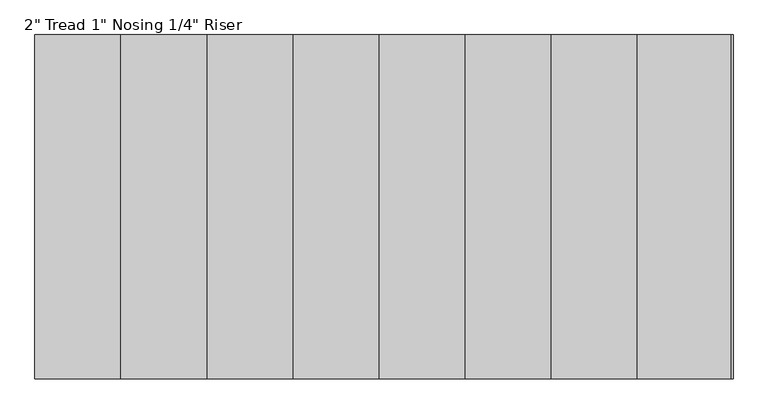
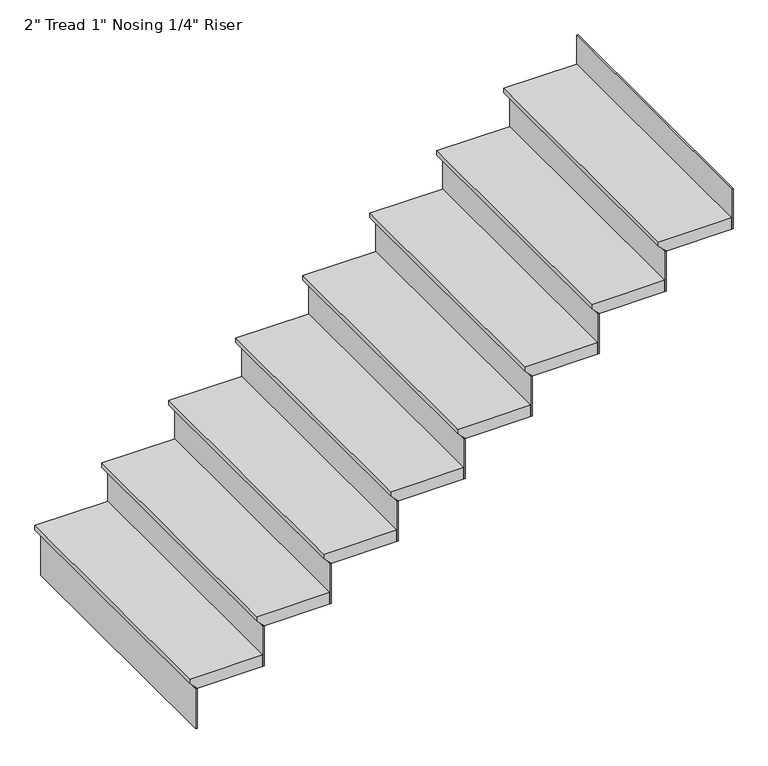
"""IFC4 building model written with IfcOpenShell, lengths in millimetres: stair flight geometry."""

from ifc_helpers import new_model, si_unit, frame, origin, place, context, project, spatial, polyline, outline, extrude, source, transform, mapped, element, save


def stair_flight_ef2f52e6(model_context):
    return source(origin(), model_context, "Body", "SweptSolid", [
        extrude(outline(polyline([(1778.0, -9891.2683044), (1778.0, -10196.0683044), (1758.95, -10196.0683044), (1733.55, -10170.6683044), (1727.2, -10170.6683044), (1727.2, -9891.2683044), (1778.0, -9891.2683044)])), frame((0.0, -2492.1891189, 0.0), z_axis=(0.0, 1.0, 0.0), x_axis=(0.0, 0.0, 1.0)), (0.0, 0.0, 1.0), 1117.6),
        extrude(outline(polyline([(-10164.3183044, -2492.1891189), (-10170.6683044, -2492.1891189), (-10170.6683044, -1374.5891189), (-10164.3183044, -1374.5891189), (-10164.3183044, -2492.1891189)])), frame((0.0, 0.0, 1549.4), z_axis=(0.0, 0.0, 1.0), x_axis=(1.0, 0.0, 0.0)), (0.0, 0.0, 1.0), 177.8),
        extrude(outline(polyline([(-9884.9183044, -2492.1891189), (-9891.2683044, -2492.1891189), (-9891.2683044, -1374.5891189), (-9884.9183044, -1374.5891189), (-9884.9183044, -2492.1891189)])), frame((0.0, 0.0, 1727.2), z_axis=(0.0, 0.0, 1.0), x_axis=(1.0, 0.0, 0.0)), (0.0, 0.0, 1.0), 177.8),
        extrude(outline(polyline([(1955.8, -9611.8683044), (1955.8, -9916.6683044), (1936.75, -9916.6683044), (1911.35, -9891.2683044), (1905.0, -9891.2683044), (1905.0, -9611.8683044), (1955.8, -9611.8683044)])), frame((0.0, -2492.1891189, 0.0), z_axis=(0.0, 1.0, 0.0), x_axis=(0.0, 0.0, 1.0)), (0.0, 0.0, 1.0), 1117.6),
        extrude(outline(polyline([(-9605.5183044, -2492.1891189), (-9611.8683044, -2492.1891189), (-9611.8683044, -1374.5891189), (-9605.5183044, -1374.5891189), (-9605.5183044, -2492.1891189)])), frame((0.0, 0.0, 1905.0), z_axis=(0.0, 0.0, 1.0), x_axis=(1.0, 0.0, 0.0)), (0.0, 0.0, 1.0), 177.8),
        extrude(outline(polyline([(2133.6, -9332.4683044), (2133.6, -9637.2683044), (2114.55, -9637.2683044), (2089.15, -9611.8683044), (2082.8, -9611.8683044), (2082.8, -9332.4683044), (2133.6, -9332.4683044)])), frame((0.0, -2492.1891189, 0.0), z_axis=(0.0, 1.0, 0.0), x_axis=(0.0, 0.0, 1.0)), (0.0, 0.0, 1.0), 1117.6),
        extrude(outline(polyline([(-9326.1183044, -2492.1891189), (-9332.4683044, -2492.1891189), (-9332.4683044, -1374.5891189), (-9326.1183044, -1374.5891189), (-9326.1183044, -2492.1891189)])), frame((0.0, 0.0, 2082.8), z_axis=(0.0, 0.0, 1.0), x_axis=(1.0, 0.0, 0.0)), (0.0, 0.0, 1.0), 177.8),
        extrude(outline(polyline([(2311.4, -9053.0683044), (2311.4, -9357.8683044), (2292.35, -9357.8683044), (2266.95, -9332.4683044), (2260.6, -9332.4683044), (2260.6, -9053.0683044), (2311.4, -9053.0683044)])), frame((0.0, -2492.1891189, 0.0), z_axis=(0.0, 1.0, 0.0), x_axis=(0.0, 0.0, 1.0)), (0.0, 0.0, 1.0), 1117.6),
        extrude(outline(polyline([(-9046.7183044, -2492.1891189), (-9053.0683044, -2492.1891189), (-9053.0683044, -1374.5891189), (-9046.7183044, -1374.5891189), (-9046.7183044, -2492.1891189)])), frame((0.0, 0.0, 2260.6), z_axis=(0.0, 0.0, 1.0), x_axis=(1.0, 0.0, 0.0)), (0.0, 0.0, 1.0), 177.8),
        extrude(outline(polyline([(2489.2, -8773.6683044), (2489.2, -9078.4683044), (2470.15, -9078.4683044), (2444.75, -9053.0683044), (2438.4, -9053.0683044), (2438.4, -8773.6683044), (2489.2, -8773.6683044)])), frame((0.0, -2492.1891189, 0.0), z_axis=(0.0, 1.0, 0.0), x_axis=(0.0, 0.0, 1.0)), (0.0, 0.0, 1.0), 1117.6),
        extrude(outline(polyline([(-8767.3183044, -2492.1891189), (-8773.6683044, -2492.1891189), (-8773.6683044, -1374.5891189), (-8767.3183044, -1374.5891189), (-8767.3183044, -2492.1891189)])), frame((0.0, 0.0, 2438.4), z_axis=(0.0, 0.0, 1.0), x_axis=(1.0, 0.0, 0.0)), (0.0, 0.0, 1.0), 177.8),
        extrude(outline(polyline([(2667.0, -8494.2683044), (2667.0, -8799.0683044), (2647.95, -8799.0683044), (2622.55, -8773.6683044), (2616.2, -8773.6683044), (2616.2, -8494.2683044), (2667.0, -8494.2683044)])), frame((0.0, -2492.1891189, 0.0), z_axis=(0.0, 1.0, 0.0), x_axis=(0.0, 0.0, 1.0)), (0.0, 0.0, 1.0), 1117.6),
        extrude(outline(polyline([(-8487.9183044, -2492.1891189), (-8494.2683044, -2492.1891189), (-8494.2683044, -1374.5891189), (-8487.9183044, -1374.5891189), (-8487.9183044, -2492.1891189)])), frame((0.0, 0.0, 2616.2), z_axis=(0.0, 0.0, 1.0), x_axis=(1.0, 0.0, 0.0)), (0.0, 0.0, 1.0), 177.8),
        extrude(outline(polyline([(2844.8, -8214.8683044), (2844.8, -8519.6683044), (2825.75, -8519.6683044), (2800.35, -8494.2683044), (2794.0, -8494.2683044), (2794.0, -8214.8683044), (2844.8, -8214.8683044)])), frame((0.0, -2492.1891189, 0.0), z_axis=(0.0, 1.0, 0.0), x_axis=(0.0, 0.0, 1.0)), (0.0, 0.0, 1.0), 1117.6),
        extrude(outline(polyline([(-8208.5183044, -2492.1891189), (-8214.8683044, -2492.1891189), (-8214.8683044, -1374.5891189), (-8208.5183044, -1374.5891189), (-8208.5183044, -2492.1891189)])), frame((0.0, 0.0, 2794.0), z_axis=(0.0, 0.0, 1.0), x_axis=(1.0, 0.0, 0.0)), (0.0, 0.0, 1.0), 177.8),
        extrude(outline(polyline([(-7929.1183044, -2492.1891189), (-7935.4683044, -2492.1891189), (-7935.4683044, -1374.5891189), (-7929.1183044, -1374.5891189), (-7929.1183044, -2492.1891189)])), frame((0.0, 0.0, 2971.8), z_axis=(0.0, 0.0, 1.0), x_axis=(1.0, 0.0, 0.0)), (0.0, 0.0, 1.0), 177.8),
        extrude(outline(polyline([(3022.6, -7935.4683044), (3022.6, -8240.2683044), (3003.55, -8240.2683044), (2978.15, -8214.8683044), (2971.8, -8214.8683044), (2971.8, -7935.4683044), (3022.6, -7935.4683044)])), frame((0.0, -2492.1891189, 0.0), z_axis=(0.0, 1.0, 0.0), x_axis=(0.0, 0.0, 1.0)), (0.0, 0.0, 1.0), 1117.6),
    ])


if __name__ == "__main__":
    model = new_model("IFC4")
    model_context = context("Model", 3, world=origin())
    ifc_project = project(units=[si_unit("LENGTHUNIT", "METRE", prefix="MILLI")], contexts=[model_context])
    site = spatial("IfcSite", under=ifc_project)
    building = spatial("IfcBuilding", under=site)
    placement = place(None, origin())
    stair_flight_shape = stair_flight_ef2f52e6(model_context)
    element("IfcStairFlight", 1, ObjectType="2\" Tread 1\" Nosing 1/4\" Riser", at=placement, inside=building, context=model_context, shape_type="MappedRepresentation", body=[
        mapped(stair_flight_shape, transform((0.0, 0.0, 0.0), x_axis=(1.0, 0.0, 0.0), y_axis=(0.0, 1.0, 0.0), z_axis=(0.0, 0.0, 1.0))),
    ])
    save(model, "model.ifc")
